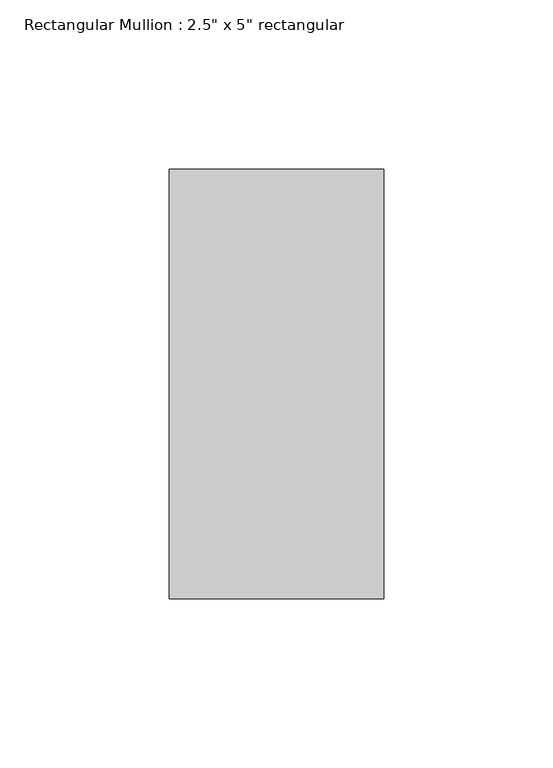
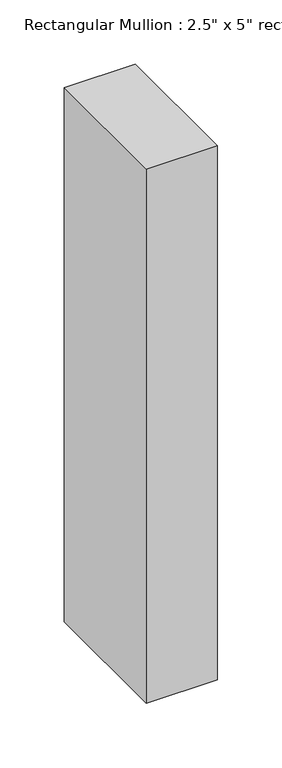
"""IFC4 building model written with IfcOpenShell, lengths in millimetres: member geometry."""

from ifc_helpers import new_model, si_unit, frame, origin, place, context, project, spatial, polyline, outline, extrude, source, transform, mapped, element, save


def member_07406574(model_context):
    return source(origin(), model_context, "Body", "SweptSolid", [
        extrude(outline(polyline([(0.0, 63.5), (0.0, -63.5), (-63.5, -63.5), (-63.5, 63.5), (0.0, 63.5)])), frame((0.0, 0.0, -505.8833333), z_axis=(0.0, 0.0, 1.0), x_axis=(1.0, 0.0, 0.0)), (0.0, 0.0, 1.0), 505.8833333),
    ])


if __name__ == "__main__":
    model = new_model("IFC4")
    model_context = context("Model", 3, world=origin())
    ifc_project = project(units=[si_unit("LENGTHUNIT", "METRE", prefix="MILLI")], contexts=[model_context])
    site = spatial("IfcSite", under=ifc_project)
    building = spatial("IfcBuilding", under=site)
    placement = place(None, origin())
    member_shape = member_07406574(model_context)
    element("IfcMember", 1, ObjectType="Rectangular Mullion : 2.5\" x 5\" rectangular", at=placement, inside=building, context=model_context, shape_type="MappedRepresentation", body=[
        mapped(member_shape, transform((0.0, 0.0, 0.0), x_axis=(1.0, 0.0, 0.0), y_axis=(0.0, 1.0, 0.0), z_axis=(0.0, 0.0, 1.0))),
    ])
    save(model, "model.ifc")

# Revit data of these elements
# Type "Rectangular Mullion : 2.5\" x 5\" rectangular"
#   built-in parameter 1007304 = 0.416667 (stored number, unit not read)
#   built-in parameter 1007301 = 0.104167 (stored number, unit not read)
#   built-in parameter 1007300 = 0.104167 (stored number, unit not read)
# Element 1 (IfcMember, "Rectangular Mullion : 2.5\" x 5\" rectangular")
#   Materials on its faces: "Aluminum"
# Materials
#   "Aluminum": class "Metal", colour RGB 247 247 247, transparency 0, Description = "Aluminum 6061", Cost = 0
